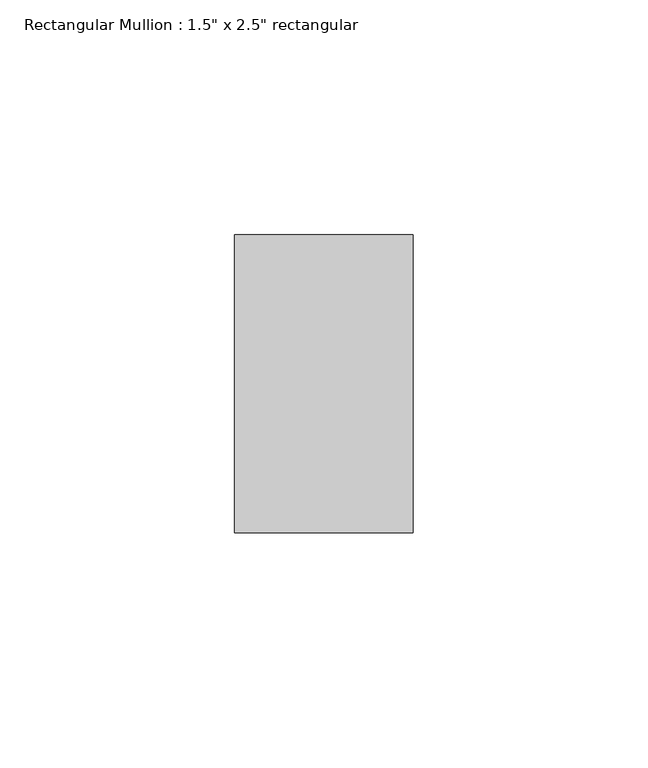
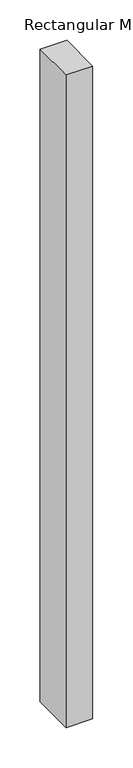
"""IFC4 building model written with IfcOpenShell, lengths in millimetres: member geometry."""

from ifc_helpers import new_model, si_unit, frame, origin, place, context, project, spatial, polyline, outline, extrude, source, transform, mapped, element, save


def member_2967a2d8(model_context):
    return source(origin(), model_context, "Body", "SweptSolid", [
        extrude(outline(polyline([(19.05, 31.75), (19.05, -31.75), (-19.05, -31.75), (-19.05, 31.75), (19.05, 31.75)])), frame((0.0, 0.0, -984.25), z_axis=(0.0, 0.0, 1.0), x_axis=(1.0, 0.0, 0.0)), (0.0, 0.0, 1.0), 984.25),
    ])


if __name__ == "__main__":
    model = new_model("IFC4")
    model_context = context("Model", 3, world=origin())
    ifc_project = project(units=[si_unit("LENGTHUNIT", "METRE", prefix="MILLI")], contexts=[model_context])
    site = spatial("IfcSite", under=ifc_project)
    building = spatial("IfcBuilding", under=site)
    placement = place(None, origin())
    member_shape = member_2967a2d8(model_context)
    element("IfcMember", 1, ObjectType="Rectangular Mullion : 1.5\" x 2.5\" rectangular", at=placement, inside=building, context=model_context, shape_type="MappedRepresentation", body=[
        mapped(member_shape, transform((0.0, 0.0, 0.0), x_axis=(1.0, 0.0, 0.0), y_axis=(0.0, 1.0, 0.0), z_axis=(0.0, 0.0, 1.0))),
    ])
    save(model, "model.ifc")

# Revit data of these elements
# Type "Rectangular Mullion : 1.5\" x 2.5\" rectangular"
#   built-in parameter 1007304 = 0.208333 (stored number, unit not read)
#   built-in parameter 1007301 = 0.0625 (stored number, unit not read)
#   built-in parameter 1007300 = 0.0625 (stored number, unit not read)
# Element 1 (IfcMember, "Rectangular Mullion : 1.5\" x 2.5\" rectangular")
#   Materials on its faces: "Aluminum"
# Materials
#   "Aluminum": class "Metal", colour RGB 247 247 247, transparency 0, Description = "Aluminum 6061", Cost = 0
